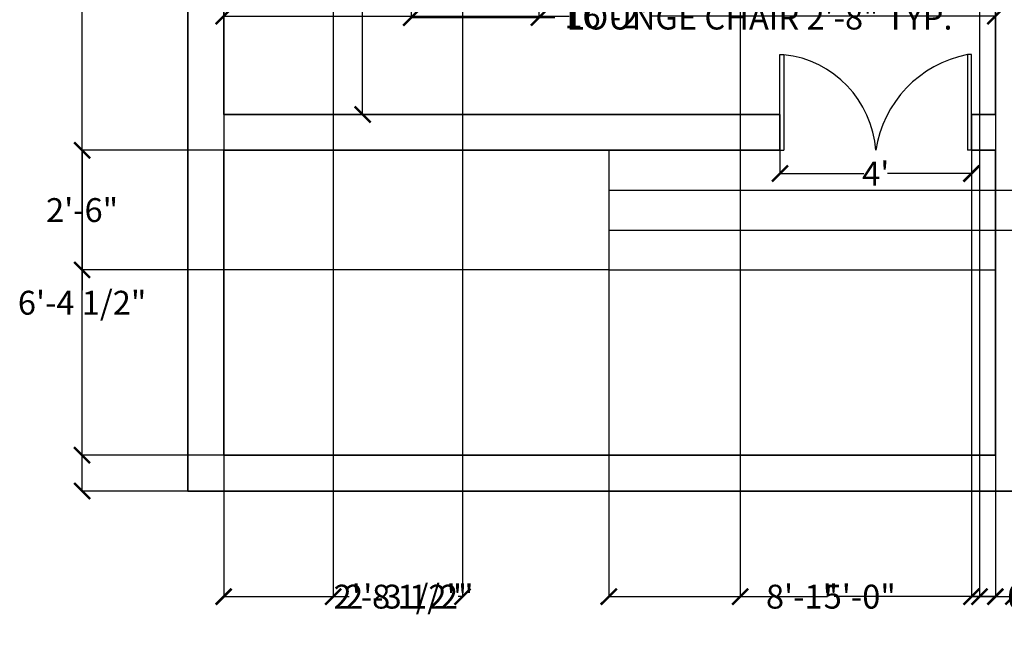
# Model space of a CAD drawing. Units: inches. Extents: x 43 to 543, y 36 to 629.
# Tile 1 of 5: x 43 to 290, y 36 to 189. Entities that reach past the tile are written whole.
import ezdxf

# ---------------------------------------------------------------- set-up
doc = ezdxf.new("R2010")
doc.units = ezdxf.units.IN
doc.header["$MEASUREMENT"] = 0
for name, color, linetype, lineweight in [('A-ANNO-DIMS', 2, 'Continuous', 18), ('A-DOOR', 3, 'Continuous', 25), ('A-FLOR-STRS', 7, 'Continuous', 25), ('A-WALL', 7, 'Continuous', 35)]:
    doc.layers.add(name, color=color, linetype=linetype, lineweight=lineweight)
doc.styles.get("Standard").update_dxf_attribs({"font": 'arial.ttf'})
doc.dimstyles.get("Standard").update_dxf_attribs({"dimtxt": 6, "dimasz": 4, "dimexe": 0.18, "dimexo": 0.0625, "dimgap": 0.09, "dimtad": 0, "dimtih": 1, "dimtoh": 1, "dimdec": 0, "dimzin": 0, "dimdsep": 46, "dimlunit": 4, "dimtxsty": 'Standard', "dimblk": 'ARCHTICK', "dimcen": 0.09, "dimadec": 0, "dimazin": 0, "dimtfac": 1, "dimtdec": 0, "dimtofl": 0, "dimtmove": 0, "dimatfit": 3, "dimldrblk": 'ARCHTICK', "dimfxl": 1, "dimtolj": 1, "dimtzin": 0, "dimarcsym": 1})

# ---------------------------------------------------------------- blocks, each defined once
blk = doc.blocks.new('_ArchTick')
at = {"color": 0, "linetype": 'ByBlock', "const_width": 0.15}
blk.add_lwpolyline([(-0.5, -0.5), (0.5, 0.5)], dxfattribs=at)
blk = doc.blocks.new('*D10')
at = {"layer": 'A-ANNO-DIMS', "color": 0, "lineweight": -2, "transparency": 16777216}
for p, q in [((93.88, 165.58), (93.88, 190.33)), ((93.88, 190.15), (180.51, 190.15)), ((287.38, 190.15), (200.74, 190.15)), ((287.38, 165.58), (287.38, 190.33))]:
    blk.add_line(p, q, dxfattribs=at)
at = {"layer": 'Defpoints', "color": 0, "transparency": 16777216}
for p in [(287.38, 190.15), (93.88, 165.52), (287.38, 165.52)]:
    blk.add_point(p, dxfattribs=at)
at = {"layer": 'A-ANNO-DIMS', "color": 0, "lineweight": -2, "transparency": 16777216, "xscale": 4, "yscale": 4, "zscale": 4, "rotation": 180}
blk.add_blockref('_ArchTick', (93.88, 190.15), dxfattribs=at)
at = {"layer": 'A-ANNO-DIMS', "color": 0, "lineweight": -2, "transparency": 16777216, "xscale": 4, "yscale": 4, "zscale": 4}
blk.add_blockref('_ArchTick', (287.38, 190.15), dxfattribs=at)
at = {"layer": 'A-ANNO-DIMS', "color": 0, "transparency": 16777216, "insert": (190.63, 190.15), "char_height": 6, "attachment_point": 5}
blk.add_mtext('\\A1;16\'-2"', dxfattribs=at)
blk = doc.blocks.new('*D11')
at = {"layer": 'A-ANNO-DIMS', "color": 0, "lineweight": -2, "transparency": 16777216}
for p, q in [((93.94, 345.52), (128.91, 345.52)), ((128.73, 345.52), (128.73, 258.67)), ((128.73, 165.52), (128.73, 252.36)), ((93.94, 165.52), (128.91, 165.52))]:
    blk.add_line(p, q, dxfattribs=at)
at = {"layer": 'Defpoints', "color": 0, "transparency": 16777216}
for p in [(93.88, 345.52), (128.73, 345.52), (93.88, 165.52)]:
    blk.add_point(p, dxfattribs=at)
at = {"layer": 'A-ANNO-DIMS', "color": 0, "lineweight": -2, "transparency": 16777216, "xscale": 4, "yscale": 4, "zscale": 4}
for p, rotation in [((128.73, 345.52), 90), ((128.73, 165.52), 270)]:
    blk.add_blockref('_ArchTick', p, dxfattribs=dict(at, rotation=rotation))
at = {"layer": 'A-ANNO-DIMS', "color": 0, "transparency": 16777216, "insert": (128.73, 255.52), "char_height": 6, "attachment_point": 5}
blk.add_mtext("\\A1;15'", dxfattribs=at)
blk = doc.blocks.new('*D19')
at = {"layer": 'A-ANNO-DIMS', "color": 0, "lineweight": -2, "transparency": 16777216}
for p, q in [((233.38, 156.45), (233.38, 150.5)), ((281.38, 156.45), (281.38, 150.5)), ((233.38, 150.68), (254.41, 150.68)), ((281.38, 150.68), (260.35, 150.68))]:
    blk.add_line(p, q, dxfattribs=at)
at = {"layer": 'Defpoints', "color": 0, "transparency": 16777216}
for p in [(233.38, 156.52), (281.38, 156.52), (281.38, 150.68)]:
    blk.add_point(p, dxfattribs=at)
at = {"layer": 'A-ANNO-DIMS', "color": 0, "lineweight": -2, "transparency": 16777216, "xscale": 4, "yscale": 4, "zscale": 4, "rotation": 180}
blk.add_blockref('_ArchTick', (233.38, 150.68), dxfattribs=at)
at = {"layer": 'A-ANNO-DIMS', "color": 0, "lineweight": -2, "transparency": 16777216, "xscale": 4, "yscale": 4, "zscale": 4}
blk.add_blockref('_ArchTick', (281.38, 150.68), dxfattribs=at)
at = {"layer": 'A-ANNO-DIMS', "color": 0, "transparency": 16777216, "insert": (257.38, 150.68), "char_height": 6, "attachment_point": 5}
blk.add_mtext("\\A1;4'", dxfattribs=at)
blk = doc.blocks.new('*D29')
at = {"layer": 'A-ANNO-DIMS', "color": 0, "lineweight": -2, "transparency": 16777216}
for p, q in [((140.89, 194.57), (140.89, 189.65)), ((172.91, 194.57), (172.91, 189.65)), ((140.89, 189.83), (172.91, 189.83)), ((172.91, 189.83), (176.91, 189.83))]:
    blk.add_line(p, q, dxfattribs=at)
at = {"layer": 'Defpoints', "color": 0, "transparency": 16777216}
for p in [(140.89, 194.63), (172.91, 194.63), (172.91, 189.83)]:
    blk.add_point(p, dxfattribs=at)
at = {"layer": 'A-ANNO-DIMS', "color": 0, "lineweight": -2, "transparency": 16777216, "xscale": 4, "yscale": 4, "zscale": 4, "rotation": 180}
blk.add_blockref('_ArchTick', (140.89, 189.83), dxfattribs=at)
at = {"layer": 'A-ANNO-DIMS', "color": 0, "lineweight": -2, "transparency": 16777216, "xscale": 4, "yscale": 4, "zscale": 4}
blk.add_blockref('_ArchTick', (172.91, 189.83), dxfattribs=at)
at = {"layer": 'A-ANNO-DIMS', "color": 0, "transparency": 16777216, "insert": (228.22, 189.83), "char_height": 6, "attachment_point": 5}
blk.add_mtext('\\A1;LOUNGE CHAIR 2\'-8" TYP.', dxfattribs=at)
blk = doc.blocks.new('*D38')
at = {"layer": 'A-ANNO-DIMS', "color": 0, "lineweight": -2, "transparency": 16777216}
for p, q in [((84.82, 599.02), (58.2, 599.02)), ((58.38, 599.02), (58.38, 338.17)), ((58.38, 71.02), (58.38, 331.86)), ((84.82, 71.02), (58.2, 71.02))]:
    blk.add_line(p, q, dxfattribs=at)
at = {"layer": 'Defpoints', "color": 0, "transparency": 16777216}
for p in [(58.38, 599.02), (84.88, 599.02), (84.88, 71.02)]:
    blk.add_point(p, dxfattribs=at)
at = {"layer": 'A-ANNO-DIMS', "color": 0, "lineweight": -2, "transparency": 16777216, "xscale": 4, "yscale": 4, "zscale": 4}
for p, rotation in [((58.38, 599.02), 90), ((58.38, 71.02), 270)]:
    blk.add_blockref('_ArchTick', p, dxfattribs=dict(at, rotation=rotation))
at = {"layer": 'A-ANNO-DIMS', "color": 0, "transparency": 16777216, "insert": (58.38, 335.02), "char_height": 6, "attachment_point": 5}
blk.add_mtext('\\A1;44\'-0"', dxfattribs=at)
blk = doc.blocks.new('*D42')
at = {"layer": 'A-ANNO-DIMS', "color": 0, "lineweight": -2, "transparency": 16777216}
for p, q in [((281.38, 156.45), (281.38, 44.34)), ((287.38, 156.45), (287.38, 44.34)), ((281.38, 44.52), (287.38, 44.52)), ((287.38, 44.52), (291.38, 44.52))]:
    blk.add_line(p, q, dxfattribs=at)
at = {"layer": 'Defpoints', "color": 0, "transparency": 16777216}
for p in [(281.38, 156.52), (287.38, 156.52), (287.38, 44.52)]:
    blk.add_point(p, dxfattribs=at)
at = {"layer": 'A-ANNO-DIMS', "color": 0, "lineweight": -2, "transparency": 16777216, "xscale": 4, "yscale": 4, "zscale": 4, "rotation": 180}
blk.add_blockref('_ArchTick', (281.38, 44.52), dxfattribs=at)
at = {"layer": 'A-ANNO-DIMS', "color": 0, "lineweight": -2, "transparency": 16777216, "xscale": 4, "yscale": 4, "zscale": 4}
blk.add_blockref('_ArchTick', (287.38, 44.52), dxfattribs=at)
at = {"layer": 'A-ANNO-DIMS', "color": 0, "transparency": 16777216, "insert": (299.44, 44.52), "char_height": 6, "attachment_point": 5}
blk.add_mtext('\\A1;0\'-6"', dxfattribs=at)
blk = doc.blocks.new('*D43')
at = {"layer": 'A-ANNO-DIMS', "color": 0, "lineweight": -2, "transparency": 16777216}
for p, q in [((93.82, 156.52), (58.2, 156.52)), ((58.38, 156.52), (58.38, 121.46)), ((58.38, 80.02), (58.38, 115.07)), ((93.82, 80.02), (58.2, 80.02))]:
    blk.add_line(p, q, dxfattribs=at)
at = {"layer": 'Defpoints', "color": 0, "transparency": 16777216}
for p in [(93.88, 156.52), (58.38, 80.02), (93.88, 80.02)]:
    blk.add_point(p, dxfattribs=at)
at = {"layer": 'A-ANNO-DIMS', "color": 0, "lineweight": -2, "transparency": 16777216, "xscale": 4, "yscale": 4, "zscale": 4}
for p, rotation in [((58.38, 156.52), 90), ((58.38, 80.02), 270)]:
    blk.add_blockref('_ArchTick', p, dxfattribs=dict(at, rotation=rotation))
at = {"layer": 'A-ANNO-DIMS', "color": 0, "transparency": 16777216, "insert": (58.38, 118.27), "char_height": 6, "attachment_point": 5}
blk.add_mtext('\\A1;6\'-4 1/2"', dxfattribs=at)
blk = doc.blocks.new('*D44')
at = {"layer": 'A-ANNO-DIMS', "color": 0, "lineweight": -2, "transparency": 16777216}
for p, q in [((121.33, 384.5), (121.33, 44.34)), ((153.74, 384.5), (153.74, 44.34)), ((121.33, 44.52), (122.43, 44.52)), ((153.74, 44.52), (152.64, 44.52))]:
    blk.add_line(p, q, dxfattribs=at)
at = {"layer": 'Defpoints', "color": 0, "transparency": 16777216}
for p in [(121.33, 384.57), (153.74, 384.57), (153.74, 44.52)]:
    blk.add_point(p, dxfattribs=at)
at = {"layer": 'A-ANNO-DIMS', "color": 0, "lineweight": -2, "transparency": 16777216, "xscale": 4, "yscale": 4, "zscale": 4, "rotation": 180}
blk.add_blockref('_ArchTick', (121.33, 44.52), dxfattribs=at)
at = {"layer": 'A-ANNO-DIMS', "color": 0, "lineweight": -2, "transparency": 16777216, "xscale": 4, "yscale": 4, "zscale": 4}
blk.add_blockref('_ArchTick', (153.74, 44.52), dxfattribs=at)
at = {"layer": 'A-ANNO-DIMS', "color": 0, "transparency": 16777216, "insert": (137.54, 44.52), "char_height": 6, "attachment_point": 5}
blk.add_mtext('\\A1;2\'-8 1/2"', dxfattribs=at)
blk = doc.blocks.new('*D54')
at = {"layer": 'A-ANNO-DIMS', "color": 0, "lineweight": -2, "transparency": 16777216}
for p, q in [((223.38, 345.45), (223.38, 44.34)), ((283.38, 345.45), (283.38, 44.34)), ((223.38, 44.52), (245.31, 44.52)), ((283.38, 44.52), (261.44, 44.52))]:
    blk.add_line(p, q, dxfattribs=at)
at = {"layer": 'Defpoints', "color": 0, "transparency": 16777216}
for p in [(223.38, 345.52), (283.38, 345.52), (283.38, 44.52)]:
    blk.add_point(p, dxfattribs=at)
at = {"layer": 'A-ANNO-DIMS', "color": 0, "lineweight": -2, "transparency": 16777216, "xscale": 4, "yscale": 4, "zscale": 4, "rotation": 180}
blk.add_blockref('_ArchTick', (223.38, 44.52), dxfattribs=at)
at = {"layer": 'A-ANNO-DIMS', "color": 0, "lineweight": -2, "transparency": 16777216, "xscale": 4, "yscale": 4, "zscale": 4}
blk.add_blockref('_ArchTick', (283.38, 44.52), dxfattribs=at)
at = {"layer": 'A-ANNO-DIMS', "color": 0, "transparency": 16777216, "insert": (253.38, 44.52), "char_height": 6, "attachment_point": 5}
blk.add_mtext('\\A1;5\'-0"', dxfattribs=at)
blk = doc.blocks.new('*D60')
at = {"layer": 'A-ANNO-DIMS', "color": 0, "lineweight": -2, "transparency": 16777216}
for p, q in [((121.33, 384.5), (121.33, 44.34)), ((93.88, 349.95), (93.88, 44.34)), ((93.88, 44.52), (121.33, 44.52)), ((121.33, 44.52), (125.33, 44.52))]:
    blk.add_line(p, q, dxfattribs=at)
at = {"layer": 'Defpoints', "color": 0, "transparency": 16777216}
for p in [(121.33, 384.57), (93.88, 350.02), (121.33, 44.52)]:
    blk.add_point(p, dxfattribs=at)
at = {"layer": 'A-ANNO-DIMS', "color": 0, "lineweight": -2, "transparency": 16777216, "xscale": 4, "yscale": 4, "zscale": 4, "rotation": 180}
blk.add_blockref('_ArchTick', (93.88, 44.52), dxfattribs=at)
at = {"layer": 'A-ANNO-DIMS', "color": 0, "lineweight": -2, "transparency": 16777216, "xscale": 4, "yscale": 4, "zscale": 4}
blk.add_blockref('_ArchTick', (121.33, 44.52), dxfattribs=at)
at = {"layer": 'A-ANNO-DIMS', "color": 0, "transparency": 16777216, "insert": (140.43, 44.52), "char_height": 6, "attachment_point": 5}
blk.add_mtext('\\A1;2\'-3 1/2"', dxfattribs=at)
blk = doc.blocks.new('*D64')
at = {"layer": 'A-ANNO-DIMS', "color": 0, "lineweight": -2, "transparency": 16777216}
for p, q in [((190.43, 126.45), (190.43, 44.34)), ((287.38, 126.45), (287.38, 44.34)), ((190.43, 44.52), (230.83, 44.52)), ((287.38, 44.52), (246.97, 44.52))]:
    blk.add_line(p, q, dxfattribs=at)
at = {"layer": 'Defpoints', "color": 0, "transparency": 16777216}
for p in [(190.43, 126.52), (287.38, 126.52), (287.38, 44.52)]:
    blk.add_point(p, dxfattribs=at)
at = {"layer": 'A-ANNO-DIMS', "color": 0, "lineweight": -2, "transparency": 16777216, "xscale": 4, "yscale": 4, "zscale": 4, "rotation": 180}
blk.add_blockref('_ArchTick', (190.43, 44.52), dxfattribs=at)
at = {"layer": 'A-ANNO-DIMS', "color": 0, "lineweight": -2, "transparency": 16777216, "xscale": 4, "yscale": 4, "zscale": 4}
blk.add_blockref('_ArchTick', (287.38, 44.52), dxfattribs=at)
at = {"layer": 'A-ANNO-DIMS', "color": 0, "transparency": 16777216, "insert": (238.9, 44.52), "char_height": 6, "attachment_point": 5}
blk.add_mtext('\\A1;8\'-1"', dxfattribs=at)
blk = doc.blocks.new('*D65')
at = {"layer": 'A-ANNO-DIMS', "color": 0, "lineweight": -2, "transparency": 16777216}
for p, q in [((190.37, 156.52), (58.2, 156.52)), ((58.38, 156.52), (58.38, 144.67)), ((58.38, 126.52), (58.38, 138.36)), ((190.37, 126.52), (58.2, 126.52))]:
    blk.add_line(p, q, dxfattribs=at)
at = {"layer": 'Defpoints', "color": 0, "transparency": 16777216}
for p in [(58.38, 156.52), (190.43, 156.52), (190.43, 126.52)]:
    blk.add_point(p, dxfattribs=at)
at = {"layer": 'A-ANNO-DIMS', "color": 0, "lineweight": -2, "transparency": 16777216, "xscale": 4, "yscale": 4, "zscale": 4}
for p, rotation in [((58.38, 156.52), 90), ((58.38, 126.52), 270)]:
    blk.add_blockref('_ArchTick', p, dxfattribs=dict(at, rotation=rotation))
at = {"layer": 'A-ANNO-DIMS', "color": 0, "transparency": 16777216, "insert": (58.38, 141.52), "char_height": 6, "attachment_point": 5}
blk.add_mtext('\\A1;2\'-6"', dxfattribs=at)
blk = doc.blocks.new('*D66')
at = {"layer": 'A-ANNO-DIMS', "color": 0, "lineweight": -2, "transparency": 16777216}
for p, q in [((287.44, 146.52), (495.56, 146.52)), ((495.38, 146.52), (495.38, 144.67)), ((495.38, 136.52), (495.38, 138.36)), ((287.44, 136.52), (495.56, 136.52))]:
    blk.add_line(p, q, dxfattribs=at)
at = {"layer": 'Defpoints', "color": 0, "transparency": 16777216}
for p in [(287.38, 146.52), (495.38, 146.52), (287.38, 136.52)]:
    blk.add_point(p, dxfattribs=at)
at = {"layer": 'A-ANNO-DIMS', "color": 0, "lineweight": -2, "transparency": 16777216, "xscale": 4, "yscale": 4, "zscale": 4}
for p, rotation in [((495.38, 146.52), 90), ((495.38, 136.52), 270)]:
    blk.add_blockref('_ArchTick', p, dxfattribs=dict(at, rotation=rotation))
at = {"layer": 'A-ANNO-DIMS', "color": 0, "transparency": 16777216, "insert": (495.38, 141.52), "char_height": 6, "attachment_point": 5}
blk.add_mtext('\\A1;0\'-10"', dxfattribs=at)
blk = doc.blocks.new('*D67')
at = {"layer": 'A-ANNO-DIMS', "color": 0, "lineweight": -2, "transparency": 16777216}
for p, q in [((287.38, 306.45), (287.38, 44.34)), ((291.88, 306.45), (291.88, 44.34)), ((287.38, 44.52), (291.88, 44.52)), ((291.88, 44.52), (295.88, 44.52))]:
    blk.add_line(p, q, dxfattribs=at)
at = {"layer": 'Defpoints', "color": 0, "transparency": 16777216}
for p in [(287.38, 306.52), (291.88, 306.52), (291.88, 44.52)]:
    blk.add_point(p, dxfattribs=at)
at = {"layer": 'A-ANNO-DIMS', "color": 0, "lineweight": -2, "transparency": 16777216, "xscale": 4, "yscale": 4, "zscale": 4, "rotation": 180}
blk.add_blockref('_ArchTick', (287.38, 44.52), dxfattribs=at)
at = {"layer": 'A-ANNO-DIMS', "color": 0, "lineweight": -2, "transparency": 16777216, "xscale": 4, "yscale": 4, "zscale": 4}
blk.add_blockref('_ArchTick', (291.88, 44.52), dxfattribs=at)
at = {"layer": 'A-ANNO-DIMS', "color": 0, "transparency": 16777216, "insert": (310.93, 44.52), "char_height": 6, "attachment_point": 5}
blk.add_mtext('\\A1;0\'-4 1/2"', dxfattribs=at)

msp = doc.modelspace()

# ---------------------------------------------------------------- linework, layer by layer
at = {"layer": 'A-DOOR'}
for p, q in [((233.38, 156.52), (233.38, 180.52)), ((233.38, 180.52), (234.38, 180.52)), ((234.38, 180.52), (234.38, 156.52)), ((281.38, 180.52), (280.38, 180.52)), ((280.38, 180.52), (280.38, 156.52)), ((281.38, 156.52), (281.38, 180.52)), ((281.38, 165.52), (281.38, 156.52)), ((233.38, 156.52), (234.38, 156.52)), ((281.38, 156.52), (280.38, 156.52))]:
    msp.add_line(p, q, dxfattribs=at)
for centre, radius, start, end in [((231.54, 154.77), 25.9, 3.861, 83.7013), ((285.93, 152.18), 28.88, 101.0819, 171.3558)]:
    msp.add_arc(centre, radius, start, end, dxfattribs=at)
at = {"layer": 'A-FLOR-STRS'}
for p, q in [((190.43, 156.52), (190.43, 126.52)), ((190.43, 146.52), (287.38, 146.52)), ((190.43, 136.52), (287.38, 136.52)), ((190.43, 126.52), (287.38, 126.52))]:
    msp.add_line(p, q, dxfattribs=at)
at = {"layer": 'A-WALL'}
for p, q in [((84.88, 71.02), (84.88, 599.02)), ((93.88, 165.52), (93.88, 345.52)), ((287.38, 306.52), (287.38, 165.52)), ((93.88, 165.52), (233.38, 165.52)), ((233.38, 165.52), (233.38, 156.52)), ((281.38, 165.52), (281.38, 156.52)), ((281.38, 165.52), (287.38, 165.52)), ((93.88, 80.02), (93.88, 156.52)), ((93.88, 156.52), (233.38, 156.52)), ((281.38, 156.52), (287.38, 156.52)), ((287.38, 156.52), (287.38, 80.02)), ((287.38, 80.02), (93.88, 80.02)), ((468.88, 71.02), (84.88, 71.02))]:
    msp.add_line(p, q, dxfattribs=at)

# ---------------------------------------------------------------- dimensions: what is measured, and where the dimension line sits
at = {"layer": 'A-ANNO-DIMS'}
for base, p1, p2, override, picture, middle in [((58.38, 599.02), (84.88, 71.02), (84.88, 599.02), {"dimdec": 1, "dimlfac": 1, "dimrnd": 0, "dimzin": 1, "dimdsep": 46, "dimlunit": 4, "dimfrac": 2}, '*D38', (58.38, 335.02)), ((128.73, 345.52), (93.88, 165.52), (93.88, 345.52), {"dimclrd": 0, "dimclre": 0, "dimclrt": 0}, '*D11', (128.73, 255.52)), ((58.38, 80.02), (93.88, 156.52), (93.88, 80.02), {"dimdec": 1, "dimlfac": 1, "dimrnd": 0, "dimzin": 1, "dimdsep": 46, "dimlunit": 4, "dimfrac": 2}, '*D43', (58.38, 118.27)), ((58.38, 156.52), (190.43, 126.52), (190.43, 156.52), {"dimdec": 1, "dimlfac": 1, "dimrnd": 0, "dimzin": 1, "dimdsep": 46, "dimlunit": 4, "dimfrac": 2}, '*D65', (58.38, 141.52)), ((495.38, 146.52), (287.38, 136.52), (287.38, 146.52), {"dimdec": 1, "dimlfac": 1, "dimrnd": 0, "dimzin": 1, "dimdsep": 46, "dimlunit": 4, "dimfrac": 2}, '*D66', (495.38, 141.52))]:
    dim = msp.add_linear_dim(base=base, p1=p1, p2=p2, angle=90, dimstyle='Standard', override=override, dxfattribs=at)
    dim.commit()
    dim.dimension.update_dxf_attribs({"geometry": picture, "text_midpoint": middle})
for base, p1, p2, override, picture, middle in [((121.3278, 44.5166), (93.8776, 350.0166), (121.3278, 384.566), {"dimdec": 1, "dimlfac": 1, "dimrnd": 0, "dimzin": 1, "dimdsep": 46, "dimlunit": 4, "dimfrac": 2}, '*D60', (140.4341, 44.5166)), ((153.74, 44.52), (121.33, 384.57), (153.74, 384.57), {"dimdec": 1, "dimlfac": 1, "dimrnd": 0, "dimzin": 1, "dimdsep": 46, "dimlunit": 4, "dimfrac": 2}, '*D44', (137.54, 44.52)), ((283.38, 44.52), (223.38, 345.52), (283.38, 345.52), {"dimdec": 1, "dimlfac": 1, "dimrnd": 0, "dimzin": 1, "dimdsep": 46, "dimlunit": 4, "dimfrac": 2}, '*D54', (253.38, 44.52)), ((291.88, 44.52), (287.38, 306.52), (291.88, 306.52), {"dimdec": 1, "dimlfac": 1, "dimrnd": 0, "dimzin": 1, "dimdsep": 46, "dimlunit": 4, "dimfrac": 2}, '*D67', (310.93, 44.52)), ((287.377649, 190.14911306), (93.877649, 165.51657912), (287.377649, 165.51657912), {"dimclrd": 0, "dimclre": 0, "dimclrt": 0}, '*D10', (190.627649, 190.14911306)), ((281.38, 150.68), (233.38, 156.52), (281.38, 156.52), {"dimclrd": 0, "dimclre": 0, "dimclrt": 0}, '*D19', (257.38, 150.68)), ((287.38, 44.52), (281.38, 156.52), (287.38, 156.52), {"dimdec": 1, "dimlfac": 1, "dimrnd": 0, "dimzin": 1, "dimdsep": 46, "dimlunit": 4, "dimfrac": 2}, '*D42', (299.44, 44.52)), ((287.3776, 44.5166), (190.4283, 126.5166), (287.3776, 126.5166), {"dimdec": 1, "dimlfac": 1, "dimrnd": 0, "dimzin": 1, "dimdsep": 46, "dimlunit": 4, "dimfrac": 2}, '*D64', (238.903, 44.5166))]:
    dim = msp.add_linear_dim(base=base, p1=p1, p2=p2, dimstyle='Standard', override=override, dxfattribs=at)
    dim.commit()
    dim.dimension.update_dxf_attribs({"geometry": picture, "text_midpoint": middle})
dim = msp.add_linear_dim(base=(172.91, 189.83), p1=(140.89, 194.63), p2=(172.91, 194.63), text='LOUNGE CHAIR <> TYP.', dimstyle='Standard', override={"dimdec": 1, "dimlfac": 1, "dimrnd": 0, "dimzin": 1, "dimdsep": 46, "dimlunit": 4, "dimfrac": 2}, dxfattribs=at)
dim.commit()
dim.dimension.update_dxf_attribs({"geometry": '*D29', "text_midpoint": (228.22, 189.83)})

doc.saveas('drawing.dxf')
